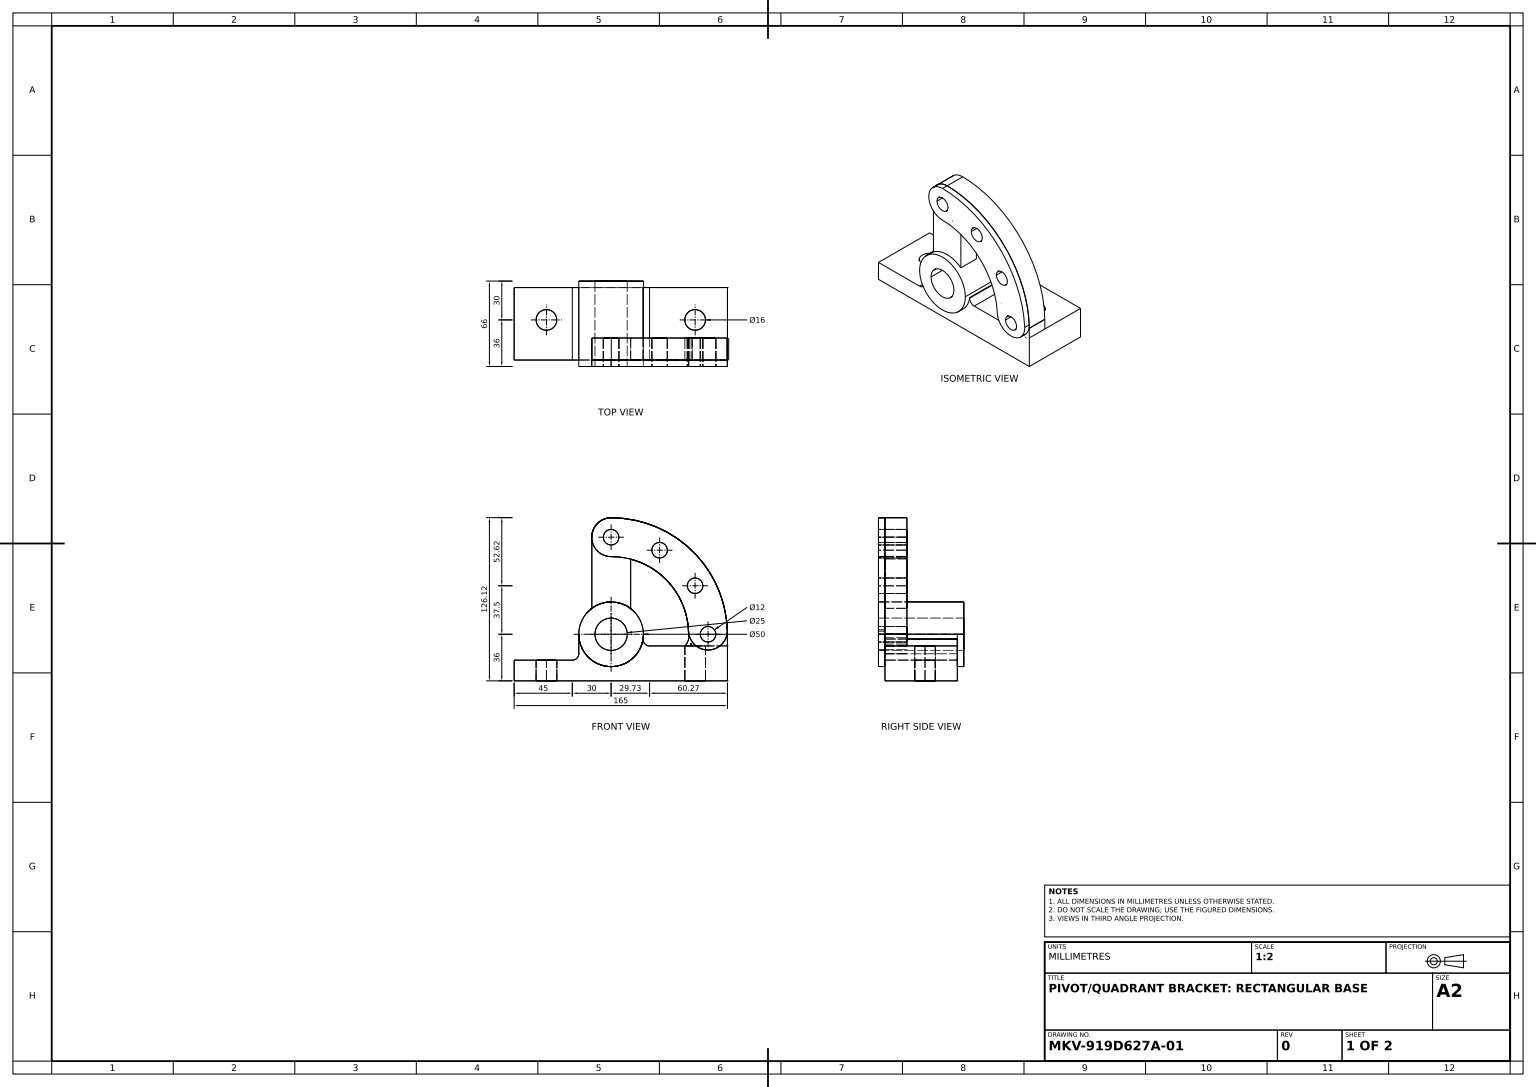
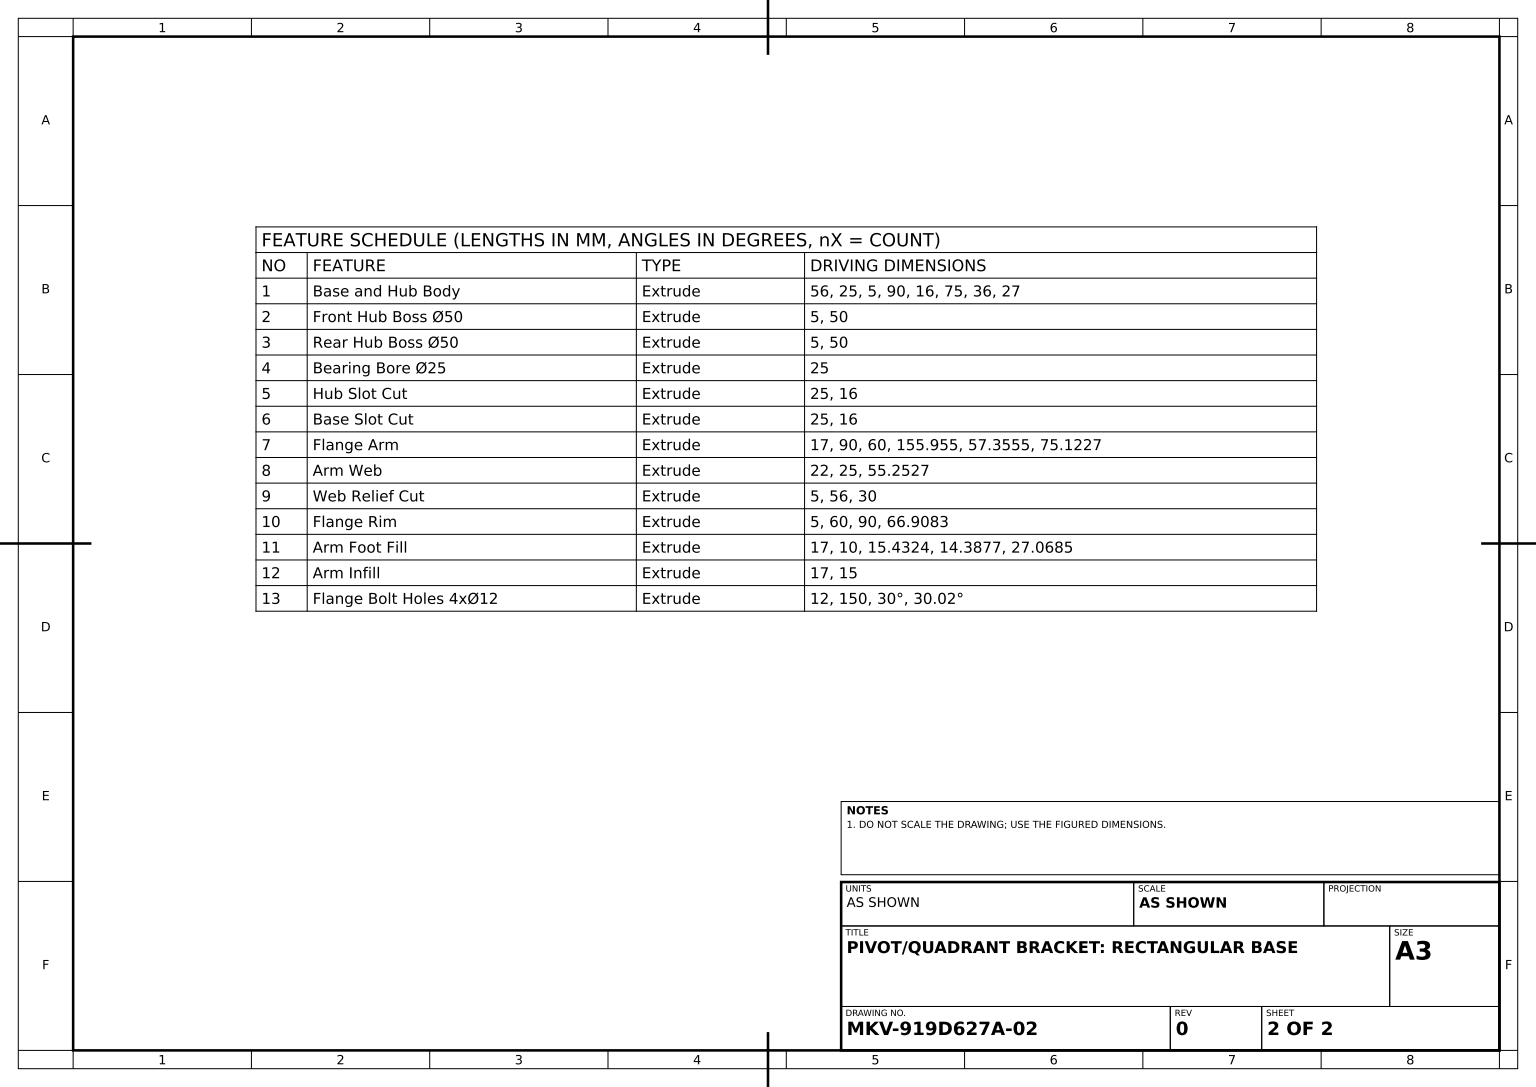
from build123d import *
from build123d.topology import SkipClean

# Parameters (mm, degrees)
BASE_AND_HUB_BODY_DEPTH       = 28
FRONT_START                   = 5
FRONT_HUB_BOSS_SKETCH_R       = 25
FRONT_HUB_BOSS_50_DEPTH       = 5
REAR_HUB_BOSS_SKETCH_R        = 25
REAR_HUB_BOSS_50_DEPTH        = 5
BEARING_BORE_SKETCH_R         = 12.5
BEARING_BORE_25_DEPTH         = 188.888264668
HUB_SLOT_SKETCH_R             = 8
HUB_SLOT_CUT_DEPTH            = 175.180940404
BASE_SLOT_SKETCH_R            = 8
BASE_SLOT_CUT_DEPTH           = 172.668284782
FLANGE_ARM_DEPTH              = 17
ARM_WEB_DEPTH                 = 22
WEB_RELIEF_CUT_DEPTH          = 5
FLANGE_RIM_DEPTH              = 5
ARM_FOOT_FILL_DEPTH           = 17
ARM_INFILL_DEPTH              = 17
FLANGE_BOLT_HOLES_SKETCH_R    = 6
FLANGE_BOLT_HOLES_4X_12_DEPTH = 218.917293143


with BuildPart() as part:
    # Base and Hub Profile Sketch → Base and Hub Body (new, symmetric)
    with BuildSketch(Plane.XY):
        with BuildLine():
            Line((0, 0), (165, 0))
            Line((165, 0), (165, 27))
            Line((165, 27), (104.732137495, 27))
            ThreePointArc((104.732137495, 27), (100.968274231, 28.708597057), (99.776781246, 32.666666667))
            ThreePointArc((99.776781246, 32.666666667), (76.670399482, 60.944132889), (50, 36))
            Line((50, 36), (50, 21))
            ThreePointArc((50, 21), (48.535533906, 17.464466094), (45, 16))
            Line((45, 16), (0, 16))
            Line((0, 16), (0, 0))
        make_face()
    extrude(amount=BASE_AND_HUB_BODY_DEPTH, both=True)

    # Front Hub Boss Sketch → Front Hub Boss Ø50 (add)
    with BuildSketch(Plane.XY.offset(28).offset(FRONT_START)):
        with Locations(Location((75, 36, 0), (0, 0, 180))):
            Circle(FRONT_HUB_BOSS_SKETCH_R)
    extrude(amount=-FRONT_HUB_BOSS_50_DEPTH)

    # Rear Hub Boss Sketch → Rear Hub Boss Ø50 (add)
    with SkipClean():  # the faces are left unmerged after this step: merging them gives an invalid solid
        with BuildSketch(Plane(origin=(0, 0, -28), x_dir=(-1, 0, 0), z_dir=(0, 0, -1))):
            with Locations((-75, 36)):
                Circle(REAR_HUB_BOSS_SKETCH_R)
        extrude(amount=REAR_HUB_BOSS_50_DEPTH)

    # Bearing Bore Sketch → Bearing Bore Ø25 (cut, through all)
    with SkipClean():  # the faces are left unmerged after this step: merging them gives an invalid solid
        with BuildSketch(Plane.XY.offset(33)):
            with Locations((75, 36)):
                Circle(BEARING_BORE_SKETCH_R)
        extrude(amount=-BEARING_BORE_25_DEPTH, mode=Mode.SUBTRACT)

    # Hub Slot Sketch → Hub Slot Cut (cut, through all)
    with SkipClean():  # the faces are left unmerged after this step: merging them gives an invalid solid
        with BuildSketch(Plane(origin=(0, 16, 0), x_dir=(1, 0, 0), z_dir=(0, 1, 0))):
            with Locations(Location((25, 3, 0), (0, 0, 270))):
                Circle(HUB_SLOT_SKETCH_R)
        extrude(amount=-HUB_SLOT_CUT_DEPTH, mode=Mode.SUBTRACT)

    # Base Slot Sketch → Base Slot Cut (cut, through all)
    with SkipClean():  # the faces are left unmerged after this step: merging them gives an invalid solid
        with BuildSketch(Plane(origin=(0, 27, 0), x_dir=(1, 0, 0), z_dir=(0, 1, 0))):
            with Locations(Location((140, 3, 0), (0, 0, 180))):
                Circle(BASE_SLOT_SKETCH_R)
        extrude(amount=-BASE_SLOT_CUT_DEPTH, mode=Mode.SUBTRACT)

    # Flange Arm Sketch → Flange Arm (add)
    with SkipClean():  # the faces are left unmerged after this step: merging them gives an invalid solid
        with BuildSketch(Plane.XY.offset(28)):
            with BuildLine():
                ThreePointArc((164.887685495, 35.975383738), (138.674843146, 99.614923148), (75.157577255, 126.122676998))
                ThreePointArc((75.157577255, 126.122676998), (60.112682879, 111.167706145), (75.067653733, 96.122811769))
                ThreePointArc((75.067653733, 96.122811769), (117.41249766, 78.450975869), (134.887725893, 36.024616262))
                ThreePointArc((134.887725893, 36.024616262), (149.863089432, 21.000020199), (164.887685495, 35.975383738))
            make_face()
        extrude(amount=-FLANGE_ARM_DEPTH)

    # Arm Web Sketch → Arm Web (add)
    with SkipClean():  # the faces are left unmerged after this step: merging them gives an invalid solid
        with BuildSketch(Plane.XY.offset(33)):
            with BuildLine():
                Line((90.112682879, 111.167706145), (60.112682879, 111.167706145))
                Line((60.112682879, 111.167706145), (60.112682879, 56.084018247))
                ThreePointArc((60.112682879, 56.084018247), (75.140854857, 60.999603195), (90.112682879, 55.914989736))
                Line((90.112682879, 55.914989736), (90.112682879, 111.167706145))
            make_face()
        extrude(amount=-ARM_WEB_DEPTH)

    # Web Relief Sketch → Web Relief Cut (cut)
    with SkipClean():  # the faces are left unmerged after this step: merging them gives an invalid solid
        with BuildSketch(Plane.XY.offset(33)):
            with BuildLine():
                Line((60.112682879, 56.084018247), (60.112682879, 112.084018247))
                Line((60.112682879, 112.084018247), (90.112682879, 112.084018247))
                Line((90.112682879, 112.084018247), (90.112682879, 55.914989736))
                ThreePointArc((90.112682879, 55.914989736), (75.140854857, 60.999603195), (60.112682879, 56.084018247))
            make_face()
        extrude(amount=-WEB_RELIEF_CUT_DEPTH, mode=Mode.SUBTRACT)

    # Flange Rim Sketch → Flange Rim (add)
    with SkipClean():  # the faces are left unmerged after this step: merging them gives an invalid solid
        with BuildSketch(Plane.XY.offset(28)):
            with BuildLine():
                ThreePointArc((164.935672679, 39.402172812), (137.425172995, 100.831302444), (75, 126))
                ThreePointArc((75, 126), (60, 111), (75, 96))
                ThreePointArc((75, 96), (116.616781997, 79.220868296), (134.957115119, 38.268115208))
                ThreePointArc((134.957115119, 38.268115208), (150.513422701, 23.84586523), (164.935672679, 39.402172812))
            make_face()
        extrude(amount=FLANGE_RIM_DEPTH)

    # Arm Foot Fill Sketch → Arm Foot Fill (add)
    with SkipClean():  # the faces are left unmerged after this step: merging them gives an invalid solid
        with BuildSketch(Plane.XY.offset(28)):
            with BuildLine():
                ThreePointArc((135.089588319, 33.547303087), (134.158093135, 29.984243626), (132, 27))
                Line((132, 27), (137.819213879, 27))
                ThreePointArc((137.819213879, 27), (137.363665204, 27.696139518), (136.94629296, 28.415816692))
                ThreePointArc((136.94629296, 28.415816692), (135.782620766, 30.896415066), (135.089588319, 33.547303087))
            make_face()
        extrude(amount=-ARM_FOOT_FILL_DEPTH)

    # Arm Infill Sketch → Arm Infill (add)
    with SkipClean():  # the faces are left unmerged after this step: merging them gives an invalid solid
        with BuildSketch(Plane.XY.offset(28)):
            with BuildLine():
                Line((161.887705694, 27), (165, 27))
                Line((165, 27), (164.887685495, 35.975383738))
                ThreePointArc((164.887685495, 35.975383738), (164.1140582, 31.244908584), (161.887705694, 27))
            make_face()
        extrude(amount=-ARM_INFILL_DEPTH)

    # Flange Bolt Holes Sketch → Flange Bolt Holes 4xØ12 (cut, through all)
    with SkipClean():  # the faces are left unmerged after this step: merging them gives an invalid solid
        with BuildSketch(Plane.XY.offset(33)):
            with Locations((150, 36)):
                Circle(FLANGE_BOLT_HOLES_SKETCH_R)
            with Locations((75, 111)):
                Circle(FLANGE_BOLT_HOLES_SKETCH_R)
            with Locations((112.5, 100.951905284)):
                Circle(FLANGE_BOLT_HOLES_SKETCH_R)
            with Locations((139.951905284, 73.5)):
                Circle(FLANGE_BOLT_HOLES_SKETCH_R)
        extrude(amount=-FLANGE_BOLT_HOLES_4X_12_DEPTH, mode=Mode.SUBTRACT)


solid = part.part
